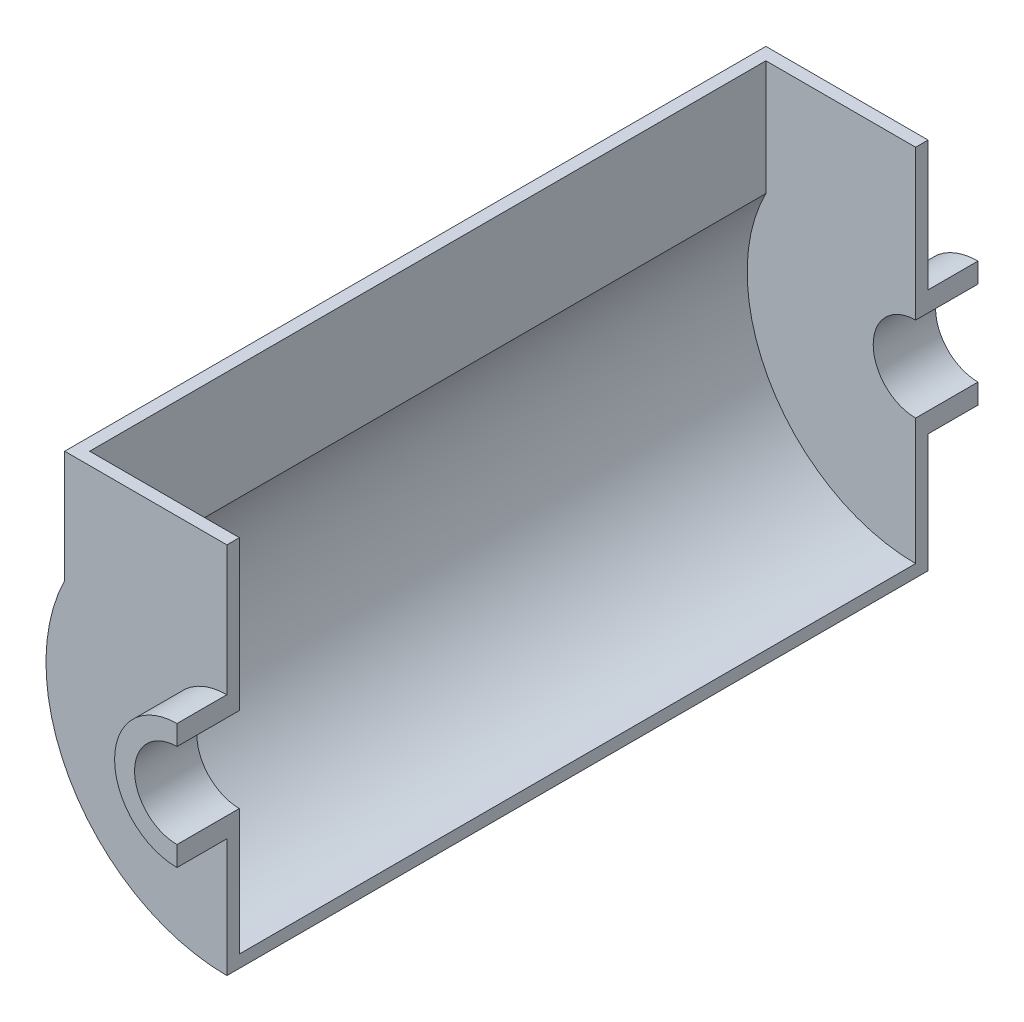
ISO-10303-21;
HEADER;
FILE_DESCRIPTION(('STEP AP214'),'2;1');
FILE_NAME('part.step','',(''),(''),'','','');
FILE_SCHEMA(('AUTOMOTIVE_DESIGN { 1 0 10303 214 1 1 1 1 }'));
ENDSEC;
DATA;
#1=APPLICATION_CONTEXT('core data for automotive mechanical design processes');
#2=APPLICATION_PROTOCOL_DEFINITION('international standard','automotive_design',2000,#1);
#3=PRODUCT_CONTEXT('',#1,'mechanical');
#4=PRODUCT('Part','Part','',(#3));
#5=PRODUCT_RELATED_PRODUCT_CATEGORY('part','',(#4));
#6=PRODUCT_DEFINITION_FORMATION('','',#4);
#7=PRODUCT_DEFINITION_CONTEXT('part definition',#1,'design');
#8=PRODUCT_DEFINITION('design','',#6,#7);
#9=PRODUCT_DEFINITION_SHAPE('','',#8);
#10=(LENGTH_UNIT() NAMED_UNIT(*) SI_UNIT(.MILLI.,.METRE.));
#11=(NAMED_UNIT(*) PLANE_ANGLE_UNIT() SI_UNIT($,.RADIAN.));
#12=(NAMED_UNIT(*) SI_UNIT($,.STERADIAN.) SOLID_ANGLE_UNIT());
#13=UNCERTAINTY_MEASURE_WITH_UNIT(LENGTH_MEASURE(1.E-05),#10,'distance_accuracy_value','');
#14=(GEOMETRIC_REPRESENTATION_CONTEXT(3) GLOBAL_UNCERTAINTY_ASSIGNED_CONTEXT((#13)) GLOBAL_UNIT_ASSIGNED_CONTEXT((#10,
#11,#12)) REPRESENTATION_CONTEXT('',''));
#15=CARTESIAN_POINT('',(0.,0.,0.));
#16=DIRECTION('',(0.,0.,1.));
#17=DIRECTION('',(1.,0.,0.));
#18=AXIS2_PLACEMENT_3D('',#15,#16,#17);
#19=CARTESIAN_POINT('',(0.,0.,-5.));
#20=DIRECTION('',(0.,0.,1.));
#21=DIRECTION('',(1.,0.,0.));
#22=AXIS2_PLACEMENT_3D('',#19,#20,#21);
#23=PLANE('',#22);
#24=CARTESIAN_POINT('',(0.,0.,-5.));
#25=DIRECTION('',(0.,0.,1.));
#26=DIRECTION('',(-1.,0.,0.));
#27=AXIS2_PLACEMENT_3D('',#24,#25,#26);
#28=CIRCLE('',#27,67.5);
#29=CARTESIAN_POINT('',(-60.,30.9232921921324,-5.));
#30=VERTEX_POINT('',#29);
#31=CARTESIAN_POINT('',(0.,-67.5,-5.));
#32=VERTEX_POINT('',#31);
#33=EDGE_CURVE('E205',#30,#32,#28,.T.);
#34=ORIENTED_EDGE('',*,*,#33,.F.);
#35=DIRECTION('',(0.,-1.,0.));
#36=VECTOR('',#35,1.);
#37=CARTESIAN_POINT('',(-60.,77.,-5.));
#38=LINE('',#37,#36);
#39=CARTESIAN_POINT('',(-60.,77.,-5.));
#40=VERTEX_POINT('',#39);
#41=EDGE_CURVE('E59',#40,#30,#38,.T.);
#42=ORIENTED_EDGE('',*,*,#41,.F.);
#43=DIRECTION('',(-1.,0.,0.));
#44=VECTOR('',#43,1.);
#45=CARTESIAN_POINT('',(0.,77.,-5.));
#46=LINE('',#45,#44);
#47=CARTESIAN_POINT('',(0.,77.,-5.));
#48=VERTEX_POINT('',#47);
#49=EDGE_CURVE('E220',#48,#40,#46,.T.);
#50=ORIENTED_EDGE('',*,*,#49,.F.);
#51=DIRECTION('',(0.,-1.,0.));
#52=VECTOR('',#51,1.);
#53=CARTESIAN_POINT('',(0.,0.,-5.));
#54=LINE('',#53,#52);
#55=CARTESIAN_POINT('',(0.,17.,-5.));
#56=VERTEX_POINT('',#55);
#57=EDGE_CURVE('E258',#48,#56,#54,.T.);
#58=ORIENTED_EDGE('',*,*,#57,.T.);
#59=CARTESIAN_POINT('',(0.,0.,-5.));
#60=DIRECTION('',(0.,0.,1.));
#61=DIRECTION('',(1.,0.,0.));
#62=AXIS2_PLACEMENT_3D('',#59,#60,#61);
#63=CIRCLE('',#62,17.);
#64=CARTESIAN_POINT('',(0.,-17.,-5.));
#65=VERTEX_POINT('',#64);
#66=EDGE_CURVE('E255',#56,#65,#63,.T.);
#67=ORIENTED_EDGE('',*,*,#66,.T.);
#68=EDGE_CURVE('E65',#65,#32,#54,.T.);
#69=ORIENTED_EDGE('',*,*,#68,.T.);
#70=EDGE_LOOP('',(#34,#42,#50,#58,#67,#69));
#71=FACE_BOUND('',#70,.T.);
#72=ADVANCED_FACE('F41',(#71),#23,.F.);
#73=CARTESIAN_POINT('',(0.,0.,-5.));
#74=DIRECTION('',(0.,0.,1.));
#75=DIRECTION('',(1.,0.,0.));
#76=AXIS2_PLACEMENT_3D('',#73,#74,#75);
#77=CYLINDRICAL_SURFACE('',#76,17.);
#78=DIRECTION('',(0.,0.,1.));
#79=VECTOR('',#78,1.);
#80=CARTESIAN_POINT('',(0.,17.,-5.));
#81=LINE('',#80,#79);
#82=CARTESIAN_POINT('',(0.,17.,20.));
#83=VERTEX_POINT('',#82);
#84=EDGE_CURVE('E44',#56,#83,#81,.T.);
#85=ORIENTED_EDGE('',*,*,#84,.T.);
#86=CARTESIAN_POINT('',(0.,0.,20.));
#87=DIRECTION('',(0.,0.,1.));
#88=DIRECTION('',(1.,0.,0.));
#89=AXIS2_PLACEMENT_3D('',#86,#87,#88);
#90=CIRCLE('',#89,17.);
#91=CARTESIAN_POINT('',(0.,-17.,20.));
#92=VERTEX_POINT('',#91);
#93=EDGE_CURVE('E239',#83,#92,#90,.T.);
#94=ORIENTED_EDGE('',*,*,#93,.T.);
#95=DIRECTION('',(0.,0.,1.));
#96=VECTOR('',#95,1.);
#97=CARTESIAN_POINT('',(0.,-17.,-5.));
#98=LINE('',#97,#96);
#99=EDGE_CURVE('E11',#65,#92,#98,.T.);
#100=ORIENTED_EDGE('',*,*,#99,.F.);
#101=ORIENTED_EDGE('',*,*,#66,.F.);
#102=EDGE_LOOP('',(#85,#94,#100,#101));
#103=FACE_BOUND('',#102,.T.);
#104=ADVANCED_FACE('F43',(#103),#77,.F.);
#105=CARTESIAN_POINT('',(0.,0.,-5.));
#106=DIRECTION('',(-1.,0.,0.));
#107=DIRECTION('',(0.,0.,1.));
#108=AXIS2_PLACEMENT_3D('',#105,#106,#107);
#109=PLANE('',#108);
#110=ORIENTED_EDGE('',*,*,#99,.T.);
#111=DIRECTION('',(0.,-1.,0.));
#112=VECTOR('',#111,1.);
#113=CARTESIAN_POINT('',(0.,0.,20.));
#114=LINE('',#113,#112);
#115=CARTESIAN_POINT('',(0.,-25.,20.));
#116=VERTEX_POINT('',#115);
#117=EDGE_CURVE('E253',#92,#116,#114,.T.);
#118=ORIENTED_EDGE('',*,*,#117,.T.);
#119=DIRECTION('',(0.,0.,1.));
#120=VECTOR('',#119,1.);
#121=CARTESIAN_POINT('',(0.,-25.,-5.));
#122=LINE('',#121,#120);
#123=CARTESIAN_POINT('',(0.,-25.,0.));
#124=VERTEX_POINT('',#123);
#125=EDGE_CURVE('E49',#124,#116,#122,.T.);
#126=ORIENTED_EDGE('',*,*,#125,.F.);
#127=DIRECTION('',(0.,1.,0.));
#128=VECTOR('',#127,1.);
#129=CARTESIAN_POINT('',(0.,-25.,0.));
#130=LINE('',#129,#128);
#131=CARTESIAN_POINT('',(0.,-72.5,0.));
#132=VERTEX_POINT('',#131);
#133=EDGE_CURVE('E219',#132,#124,#130,.T.);
#134=ORIENTED_EDGE('',*,*,#133,.F.);
#135=DIRECTION('',(0.,0.,1.));
#136=VECTOR('',#135,1.);
#137=CARTESIAN_POINT('',(0.,-72.5,-5.));
#138=LINE('',#137,#136);
#139=CARTESIAN_POINT('',(0.,-72.5,-281.));
#140=VERTEX_POINT('',#139);
#141=EDGE_CURVE('E240',#140,#132,#138,.T.);
#142=ORIENTED_EDGE('',*,*,#141,.F.);
#143=DIRECTION('',(0.,1.,0.));
#144=VECTOR('',#143,1.);
#145=CARTESIAN_POINT('',(0.,-25.,-281.));
#146=LINE('',#145,#144);
#147=CARTESIAN_POINT('',(0.,-25.,-281.));
#148=VERTEX_POINT('',#147);
#149=EDGE_CURVE('E169',#140,#148,#146,.T.);
#150=ORIENTED_EDGE('',*,*,#149,.T.);
#151=DIRECTION('',(0.,0.,-1.));
#152=VECTOR('',#151,1.);
#153=CARTESIAN_POINT('',(0.,-25.,-276.));
#154=LINE('',#153,#152);
#155=CARTESIAN_POINT('',(0.,-25.,-301.));
#156=VERTEX_POINT('',#155);
#157=EDGE_CURVE('E193',#148,#156,#154,.T.);
#158=ORIENTED_EDGE('',*,*,#157,.T.);
#159=DIRECTION('',(0.,-1.,0.));
#160=VECTOR('',#159,1.);
#161=CARTESIAN_POINT('',(0.,0.,-301.));
#162=LINE('',#161,#160);
#163=CARTESIAN_POINT('',(0.,-17.,-301.));
#164=VERTEX_POINT('',#163);
#165=EDGE_CURVE('E189',#164,#156,#162,.T.);
#166=ORIENTED_EDGE('',*,*,#165,.F.);
#167=DIRECTION('',(0.,0.,-1.));
#168=VECTOR('',#167,1.);
#169=CARTESIAN_POINT('',(0.,-17.,-276.));
#170=LINE('',#169,#168);
#171=CARTESIAN_POINT('',(0.,-17.,-276.));
#172=VERTEX_POINT('',#171);
#173=EDGE_CURVE('E191',#172,#164,#170,.T.);
#174=ORIENTED_EDGE('',*,*,#173,.F.);
#175=DIRECTION('',(0.,-1.,0.));
#176=VECTOR('',#175,1.);
#177=CARTESIAN_POINT('',(0.,0.,-276.));
#178=LINE('',#177,#176);
#179=CARTESIAN_POINT('',(0.,-67.5,-276.));
#180=VERTEX_POINT('',#179);
#181=EDGE_CURVE('E181',#172,#180,#178,.T.);
#182=ORIENTED_EDGE('',*,*,#181,.T.);
#183=DIRECTION('',(0.,0.,1.));
#184=VECTOR('',#183,1.);
#185=CARTESIAN_POINT('',(0.,-67.5,-301.002));
#186=LINE('',#185,#184);
#187=EDGE_CURVE('E202',#180,#32,#186,.T.);
#188=ORIENTED_EDGE('',*,*,#187,.T.);
#189=ORIENTED_EDGE('',*,*,#68,.F.);
#190=EDGE_LOOP('',(#110,#118,#126,#134,#142,#150,#158,#166,#174,#182,#188,#189));
#191=FACE_BOUND('',#190,.T.);
#192=ADVANCED_FACE('F280',(#191),#109,.F.);
#193=CARTESIAN_POINT('',(0.,0.,-5.));
#194=DIRECTION('',(0.,0.,1.));
#195=DIRECTION('',(1.,0.,0.));
#196=AXIS2_PLACEMENT_3D('',#193,#194,#195);
#197=CYLINDRICAL_SURFACE('',#196,25.);
#198=CARTESIAN_POINT('',(0.,0.,0.));
#199=DIRECTION('',(0.,0.,-1.));
#200=DIRECTION('',(1.,0.,0.));
#201=AXIS2_PLACEMENT_3D('',#198,#199,#200);
#202=CIRCLE('',#201,25.);
#203=CARTESIAN_POINT('',(0.,25.,0.));
#204=VERTEX_POINT('',#203);
#205=EDGE_CURVE('E214',#124,#204,#202,.T.);
#206=ORIENTED_EDGE('',*,*,#205,.F.);
#207=ORIENTED_EDGE('',*,*,#125,.T.);
#208=CARTESIAN_POINT('',(0.,0.,20.));
#209=DIRECTION('',(0.,0.,1.));
#210=DIRECTION('',(1.,0.,0.));
#211=AXIS2_PLACEMENT_3D('',#208,#209,#210);
#212=CIRCLE('',#211,25.);
#213=CARTESIAN_POINT('',(0.,25.,20.));
#214=VERTEX_POINT('',#213);
#215=EDGE_CURVE('E250',#214,#116,#212,.T.);
#216=ORIENTED_EDGE('',*,*,#215,.F.);
#217=DIRECTION('',(0.,0.,1.));
#218=VECTOR('',#217,1.);
#219=CARTESIAN_POINT('',(0.,25.,-5.));
#220=LINE('',#219,#218);
#221=EDGE_CURVE('E256',#204,#214,#220,.T.);
#222=ORIENTED_EDGE('',*,*,#221,.F.);
#223=EDGE_LOOP('',(#206,#207,#216,#222));
#224=FACE_BOUND('',#223,.T.);
#225=ADVANCED_FACE('F274',(#224),#197,.T.);
#226=ORIENTED_EDGE('',*,*,#57,.F.);
#227=DIRECTION('',(0.,0.,1.));
#228=VECTOR('',#227,1.);
#229=CARTESIAN_POINT('',(0.,77.,-5.));
#230=LINE('',#229,#228);
#231=CARTESIAN_POINT('',(0.,77.,0.));
#232=VERTEX_POINT('',#231);
#233=EDGE_CURVE('E218',#48,#232,#230,.T.);
#234=ORIENTED_EDGE('',*,*,#233,.T.);
#235=DIRECTION('',(0.,1.,0.));
#236=VECTOR('',#235,1.);
#237=CARTESIAN_POINT('',(0.,25.,0.));
#238=LINE('',#237,#236);
#239=EDGE_CURVE('E224',#204,#232,#238,.T.);
#240=ORIENTED_EDGE('',*,*,#239,.F.);
#241=ORIENTED_EDGE('',*,*,#221,.T.);
#242=EDGE_CURVE('E247',#214,#83,#114,.T.);
#243=ORIENTED_EDGE('',*,*,#242,.T.);
#244=ORIENTED_EDGE('',*,*,#84,.F.);
#245=EDGE_LOOP('',(#226,#234,#240,#241,#243,#244));
#246=FACE_BOUND('',#245,.T.);
#247=ADVANCED_FACE('F275',(#246),#109,.F.);
#248=CARTESIAN_POINT('',(0.,0.,20.));
#249=DIRECTION('',(0.,0.,1.));
#250=DIRECTION('',(1.,0.,0.));
#251=AXIS2_PLACEMENT_3D('',#248,#249,#250);
#252=PLANE('',#251);
#253=ORIENTED_EDGE('',*,*,#93,.F.);
#254=ORIENTED_EDGE('',*,*,#242,.F.);
#255=ORIENTED_EDGE('',*,*,#215,.T.);
#256=ORIENTED_EDGE('',*,*,#117,.F.);
#257=EDGE_LOOP('',(#253,#254,#255,#256));
#258=FACE_BOUND('',#257,.T.);
#259=ADVANCED_FACE('F269',(#258),#252,.T.);
#260=CARTESIAN_POINT('',(0.,0.,-5.));
#261=DIRECTION('',(0.,0.,1.));
#262=DIRECTION('',(1.,0.,0.));
#263=AXIS2_PLACEMENT_3D('',#260,#261,#262);
#264=CYLINDRICAL_SURFACE('',#263,72.5);
#265=CARTESIAN_POINT('',(0.,0.,0.));
#266=DIRECTION('',(0.,0.,1.));
#267=DIRECTION('',(1.,0.,0.));
#268=AXIS2_PLACEMENT_3D('',#265,#266,#267);
#269=CIRCLE('',#268,72.5);
#270=CARTESIAN_POINT('',(-65.,32.1130814466629,0.));
#271=VERTEX_POINT('',#270);
#272=EDGE_CURVE('E232',#271,#132,#269,.T.);
#273=ORIENTED_EDGE('',*,*,#272,.F.);
#274=DIRECTION('',(0.,0.,1.));
#275=VECTOR('',#274,1.);
#276=CARTESIAN_POINT('',(-65.,32.1130814466629,-5.));
#277=LINE('',#276,#275);
#278=CARTESIAN_POINT('',(-65.,32.1130814466629,-281.));
#279=VERTEX_POINT('',#278);
#280=EDGE_CURVE('E238',#279,#271,#277,.T.);
#281=ORIENTED_EDGE('',*,*,#280,.F.);
#282=CARTESIAN_POINT('',(0.,0.,-281.));
#283=DIRECTION('',(0.,0.,1.));
#284=DIRECTION('',(1.,0.,0.));
#285=AXIS2_PLACEMENT_3D('',#282,#283,#284);
#286=CIRCLE('',#285,72.5);
#287=EDGE_CURVE('E350',#279,#140,#286,.T.);
#288=ORIENTED_EDGE('',*,*,#287,.T.);
#289=ORIENTED_EDGE('',*,*,#141,.T.);
#290=EDGE_LOOP('',(#273,#281,#288,#289));
#291=FACE_BOUND('',#290,.T.);
#292=ADVANCED_FACE('F282',(#291),#264,.T.);
#293=CARTESIAN_POINT('',(-65.,77.,-5.));
#294=DIRECTION('',(-1.,0.,0.));
#295=DIRECTION('',(0.,-1.,0.));
#296=AXIS2_PLACEMENT_3D('',#293,#294,#295);
#297=PLANE('',#296);
#298=DIRECTION('',(0.,-1.,0.));
#299=VECTOR('',#298,1.);
#300=CARTESIAN_POINT('',(-65.,77.,0.));
#301=LINE('',#300,#299);
#302=CARTESIAN_POINT('',(-65.,77.,0.));
#303=VERTEX_POINT('',#302);
#304=EDGE_CURVE('E230',#303,#271,#301,.T.);
#305=ORIENTED_EDGE('',*,*,#304,.F.);
#306=DIRECTION('',(0.,0.,1.));
#307=VECTOR('',#306,1.);
#308=CARTESIAN_POINT('',(-65.,77.,-5.));
#309=LINE('',#308,#307);
#310=CARTESIAN_POINT('',(-65.,77.,-281.));
#311=VERTEX_POINT('',#310);
#312=EDGE_CURVE('E244',#311,#303,#309,.T.);
#313=ORIENTED_EDGE('',*,*,#312,.F.);
#314=DIRECTION('',(0.,-1.,0.));
#315=VECTOR('',#314,1.);
#316=CARTESIAN_POINT('',(-65.,77.,-281.));
#317=LINE('',#316,#315);
#318=EDGE_CURVE('E349',#311,#279,#317,.T.);
#319=ORIENTED_EDGE('',*,*,#318,.T.);
#320=ORIENTED_EDGE('',*,*,#280,.T.);
#321=EDGE_LOOP('',(#305,#313,#319,#320));
#322=FACE_BOUND('',#321,.T.);
#323=ADVANCED_FACE('F299',(#322),#297,.T.);
#324=CARTESIAN_POINT('',(0.,77.,-5.));
#325=DIRECTION('',(0.,1.,0.));
#326=DIRECTION('',(-1.,0.,0.));
#327=AXIS2_PLACEMENT_3D('',#324,#325,#326);
#328=PLANE('',#327);
#329=DIRECTION('',(-1.,0.,0.));
#330=VECTOR('',#329,1.);
#331=CARTESIAN_POINT('',(0.,77.,0.));
#332=LINE('',#331,#330);
#333=EDGE_CURVE('E228',#232,#303,#332,.T.);
#334=ORIENTED_EDGE('',*,*,#333,.F.);
#335=ORIENTED_EDGE('',*,*,#233,.F.);
#336=ORIENTED_EDGE('',*,*,#49,.T.);
#337=DIRECTION('',(0.,0.,1.));
#338=VECTOR('',#337,1.);
#339=CARTESIAN_POINT('',(-60.,77.,-301.002));
#340=LINE('',#339,#338);
#341=CARTESIAN_POINT('',(-60.,77.,-276.));
#342=VERTEX_POINT('',#341);
#343=EDGE_CURVE('E163',#342,#40,#340,.T.);
#344=ORIENTED_EDGE('',*,*,#343,.F.);
#345=DIRECTION('',(-1.,0.,0.));
#346=VECTOR('',#345,1.);
#347=CARTESIAN_POINT('',(0.,77.,-276.));
#348=LINE('',#347,#346);
#349=CARTESIAN_POINT('',(0.,77.,-276.));
#350=VERTEX_POINT('',#349);
#351=EDGE_CURVE('E156',#350,#342,#348,.T.);
#352=ORIENTED_EDGE('',*,*,#351,.F.);
#353=DIRECTION('',(0.,0.,-1.));
#354=VECTOR('',#353,1.);
#355=CARTESIAN_POINT('',(0.,77.,-276.));
#356=LINE('',#355,#354);
#357=CARTESIAN_POINT('',(0.,77.,-281.));
#358=VERTEX_POINT('',#357);
#359=EDGE_CURVE('E161',#350,#358,#356,.T.);
#360=ORIENTED_EDGE('',*,*,#359,.T.);
#361=DIRECTION('',(-1.,0.,0.));
#362=VECTOR('',#361,1.);
#363=CARTESIAN_POINT('',(0.,77.,-281.));
#364=LINE('',#363,#362);
#365=EDGE_CURVE('E365',#358,#311,#364,.T.);
#366=ORIENTED_EDGE('',*,*,#365,.T.);
#367=ORIENTED_EDGE('',*,*,#312,.T.);
#368=EDGE_LOOP('',(#334,#335,#336,#344,#352,#360,#366,#367));
#369=FACE_BOUND('',#368,.T.);
#370=ADVANCED_FACE('F157',(#369),#328,.T.);
#371=CARTESIAN_POINT('',(0.,0.,0.));
#372=DIRECTION('',(0.,0.,1.));
#373=DIRECTION('',(1.,0.,0.));
#374=AXIS2_PLACEMENT_3D('',#371,#372,#373);
#375=PLANE('',#374);
#376=ORIENTED_EDGE('',*,*,#205,.T.);
#377=ORIENTED_EDGE('',*,*,#239,.T.);
#378=ORIENTED_EDGE('',*,*,#333,.T.);
#379=ORIENTED_EDGE('',*,*,#304,.T.);
#380=ORIENTED_EDGE('',*,*,#272,.T.);
#381=ORIENTED_EDGE('',*,*,#133,.T.);
#382=EDGE_LOOP('',(#376,#377,#378,#379,#380,#381));
#383=FACE_BOUND('',#382,.T.);
#384=ADVANCED_FACE('F298',(#383),#375,.T.);
#385=CARTESIAN_POINT('',(-60.,77.,-301.002));
#386=DIRECTION('',(-1.,0.,0.));
#387=DIRECTION('',(0.,0.,1.));
#388=AXIS2_PLACEMENT_3D('',#385,#386,#387);
#389=PLANE('',#388);
#390=DIRECTION('',(0.,-1.,0.));
#391=VECTOR('',#390,1.);
#392=CARTESIAN_POINT('',(-60.,77.,-276.));
#393=LINE('',#392,#391);
#394=CARTESIAN_POINT('',(-60.,30.9232921921324,-276.));
#395=VERTEX_POINT('',#394);
#396=EDGE_CURVE('E210',#342,#395,#393,.T.);
#397=ORIENTED_EDGE('',*,*,#396,.F.);
#398=ORIENTED_EDGE('',*,*,#343,.T.);
#399=ORIENTED_EDGE('',*,*,#41,.T.);
#400=DIRECTION('',(0.,0.,1.));
#401=VECTOR('',#400,1.);
#402=CARTESIAN_POINT('',(-60.,30.9232921921324,-301.002));
#403=LINE('',#402,#401);
#404=EDGE_CURVE('E208',#395,#30,#403,.T.);
#405=ORIENTED_EDGE('',*,*,#404,.F.);
#406=EDGE_LOOP('',(#397,#398,#399,#405));
#407=FACE_BOUND('',#406,.T.);
#408=ADVANCED_FACE('F305',(#407),#389,.F.);
#409=CARTESIAN_POINT('',(0.,0.,-301.002));
#410=DIRECTION('',(0.,0.,1.));
#411=DIRECTION('',(1.,0.,0.));
#412=AXIS2_PLACEMENT_3D('',#409,#410,#411);
#413=CYLINDRICAL_SURFACE('',#412,67.5);
#414=CARTESIAN_POINT('',(0.,0.,-276.));
#415=DIRECTION('',(0.,0.,-1.));
#416=DIRECTION('',(-1.,0.,0.));
#417=AXIS2_PLACEMENT_3D('',#414,#415,#416);
#418=CIRCLE('',#417,67.5);
#419=EDGE_CURVE('E215',#395,#180,#418,.F.);
#420=ORIENTED_EDGE('',*,*,#419,.F.);
#421=ORIENTED_EDGE('',*,*,#404,.T.);
#422=ORIENTED_EDGE('',*,*,#33,.T.);
#423=ORIENTED_EDGE('',*,*,#187,.F.);
#424=EDGE_LOOP('',(#420,#421,#422,#423));
#425=FACE_BOUND('',#424,.T.);
#426=ADVANCED_FACE('F307',(#425),#413,.F.);
#427=CARTESIAN_POINT('',(0.,0.,-276.));
#428=DIRECTION('',(0.,0.,-1.));
#429=DIRECTION('',(1.,0.,0.));
#430=AXIS2_PLACEMENT_3D('',#427,#428,#429);
#431=PLANE('',#430);
#432=ORIENTED_EDGE('',*,*,#351,.T.);
#433=ORIENTED_EDGE('',*,*,#396,.T.);
#434=ORIENTED_EDGE('',*,*,#419,.T.);
#435=ORIENTED_EDGE('',*,*,#181,.F.);
#436=CARTESIAN_POINT('',(0.,0.,-276.));
#437=DIRECTION('',(0.,0.,1.));
#438=DIRECTION('',(1.,0.,0.));
#439=AXIS2_PLACEMENT_3D('',#436,#437,#438);
#440=CIRCLE('',#439,17.);
#441=CARTESIAN_POINT('',(0.,17.,-276.));
#442=VERTEX_POINT('',#441);
#443=EDGE_CURVE('E182',#442,#172,#440,.T.);
#444=ORIENTED_EDGE('',*,*,#443,.F.);
#445=EDGE_CURVE('E172',#350,#442,#178,.T.);
#446=ORIENTED_EDGE('',*,*,#445,.F.);
#447=EDGE_LOOP('',(#432,#433,#434,#435,#444,#446));
#448=FACE_BOUND('',#447,.T.);
#449=ADVANCED_FACE('F178',(#448),#431,.F.);
#450=CARTESIAN_POINT('',(0.,0.,-276.));
#451=DIRECTION('',(0.,0.,-1.));
#452=DIRECTION('',(1.,0.,0.));
#453=AXIS2_PLACEMENT_3D('',#450,#451,#452);
#454=CYLINDRICAL_SURFACE('',#453,17.);
#455=DIRECTION('',(0.,0.,-1.));
#456=VECTOR('',#455,1.);
#457=CARTESIAN_POINT('',(0.,17.,-276.));
#458=LINE('',#457,#456);
#459=CARTESIAN_POINT('',(0.,17.,-301.));
#460=VERTEX_POINT('',#459);
#461=EDGE_CURVE('E188',#442,#460,#458,.T.);
#462=ORIENTED_EDGE('',*,*,#461,.F.);
#463=ORIENTED_EDGE('',*,*,#443,.T.);
#464=ORIENTED_EDGE('',*,*,#173,.T.);
#465=CARTESIAN_POINT('',(0.,0.,-301.));
#466=DIRECTION('',(0.,0.,1.));
#467=DIRECTION('',(1.,0.,0.));
#468=AXIS2_PLACEMENT_3D('',#465,#466,#467);
#469=CIRCLE('',#468,17.);
#470=EDGE_CURVE('E177',#460,#164,#469,.T.);
#471=ORIENTED_EDGE('',*,*,#470,.F.);
#472=EDGE_LOOP('',(#462,#463,#464,#471));
#473=FACE_BOUND('',#472,.T.);
#474=ADVANCED_FACE('F314',(#473),#454,.F.);
#475=CARTESIAN_POINT('',(0.,0.,-276.));
#476=DIRECTION('',(0.,0.,-1.));
#477=DIRECTION('',(1.,0.,0.));
#478=AXIS2_PLACEMENT_3D('',#475,#476,#477);
#479=CYLINDRICAL_SURFACE('',#478,25.);
#480=CARTESIAN_POINT('',(0.,0.,-281.));
#481=DIRECTION('',(0.,0.,-1.));
#482=DIRECTION('',(1.,0.,0.));
#483=AXIS2_PLACEMENT_3D('',#480,#481,#482);
#484=CIRCLE('',#483,25.);
#485=CARTESIAN_POINT('',(0.,25.,-281.));
#486=VERTEX_POINT('',#485);
#487=EDGE_CURVE('E339',#148,#486,#484,.T.);
#488=ORIENTED_EDGE('',*,*,#487,.T.);
#489=DIRECTION('',(0.,0.,-1.));
#490=VECTOR('',#489,1.);
#491=CARTESIAN_POINT('',(0.,25.,-276.));
#492=LINE('',#491,#490);
#493=CARTESIAN_POINT('',(0.,25.,-301.));
#494=VERTEX_POINT('',#493);
#495=EDGE_CURVE('E197',#486,#494,#492,.T.);
#496=ORIENTED_EDGE('',*,*,#495,.T.);
#497=CARTESIAN_POINT('',(0.,0.,-301.));
#498=DIRECTION('',(0.,0.,1.));
#499=DIRECTION('',(1.,0.,0.));
#500=AXIS2_PLACEMENT_3D('',#497,#498,#499);
#501=CIRCLE('',#500,25.);
#502=EDGE_CURVE('E344',#494,#156,#501,.T.);
#503=ORIENTED_EDGE('',*,*,#502,.T.);
#504=ORIENTED_EDGE('',*,*,#157,.F.);
#505=EDGE_LOOP('',(#488,#496,#503,#504));
#506=FACE_BOUND('',#505,.T.);
#507=ADVANCED_FACE('F320',(#506),#479,.T.);
#508=CARTESIAN_POINT('',(0.,0.,-276.));
#509=DIRECTION('',(-1.,0.,0.));
#510=DIRECTION('',(0.,0.,-1.));
#511=AXIS2_PLACEMENT_3D('',#508,#509,#510);
#512=PLANE('',#511);
#513=ORIENTED_EDGE('',*,*,#445,.T.);
#514=ORIENTED_EDGE('',*,*,#461,.T.);
#515=EDGE_CURVE('E351',#494,#460,#162,.T.);
#516=ORIENTED_EDGE('',*,*,#515,.F.);
#517=ORIENTED_EDGE('',*,*,#495,.F.);
#518=DIRECTION('',(0.,1.,0.));
#519=VECTOR('',#518,1.);
#520=CARTESIAN_POINT('',(0.,25.,-281.));
#521=LINE('',#520,#519);
#522=EDGE_CURVE('E176',#486,#358,#521,.T.);
#523=ORIENTED_EDGE('',*,*,#522,.T.);
#524=ORIENTED_EDGE('',*,*,#359,.F.);
#525=EDGE_LOOP('',(#513,#514,#516,#517,#523,#524));
#526=FACE_BOUND('',#525,.T.);
#527=ADVANCED_FACE('F173',(#526),#512,.F.);
#528=CARTESIAN_POINT('',(0.,0.,-301.));
#529=DIRECTION('',(0.,0.,-1.));
#530=DIRECTION('',(1.,0.,0.));
#531=AXIS2_PLACEMENT_3D('',#528,#529,#530);
#532=PLANE('',#531);
#533=ORIENTED_EDGE('',*,*,#470,.T.);
#534=ORIENTED_EDGE('',*,*,#165,.T.);
#535=ORIENTED_EDGE('',*,*,#502,.F.);
#536=ORIENTED_EDGE('',*,*,#515,.T.);
#537=EDGE_LOOP('',(#533,#534,#535,#536));
#538=FACE_BOUND('',#537,.T.);
#539=ADVANCED_FACE('F322',(#538),#532,.T.);
#540=CARTESIAN_POINT('',(0.,0.,-281.));
#541=DIRECTION('',(0.,0.,-1.));
#542=DIRECTION('',(1.,0.,0.));
#543=AXIS2_PLACEMENT_3D('',#540,#541,#542);
#544=PLANE('',#543);
#545=ORIENTED_EDGE('',*,*,#487,.F.);
#546=ORIENTED_EDGE('',*,*,#149,.F.);
#547=ORIENTED_EDGE('',*,*,#287,.F.);
#548=ORIENTED_EDGE('',*,*,#318,.F.);
#549=ORIENTED_EDGE('',*,*,#365,.F.);
#550=ORIENTED_EDGE('',*,*,#522,.F.);
#551=EDGE_LOOP('',(#545,#546,#547,#548,#549,#550));
#552=FACE_BOUND('',#551,.T.);
#553=ADVANCED_FACE('F328',(#552),#544,.T.);
#554=CLOSED_SHELL('',(#72,#104,#192,#225,#247,#259,#292,#323,#370,#384,#408,#426,#449,#474,#507,
#527,#539,#553));
#555=MANIFOLD_SOLID_BREP('B2',#554);
#556=ADVANCED_BREP_SHAPE_REPRESENTATION('',(#18,#555),#14);
#557=SHAPE_DEFINITION_REPRESENTATION(#9,#556);
ENDSEC;
END-ISO-10303-21;
